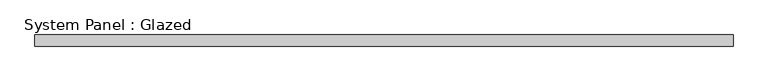
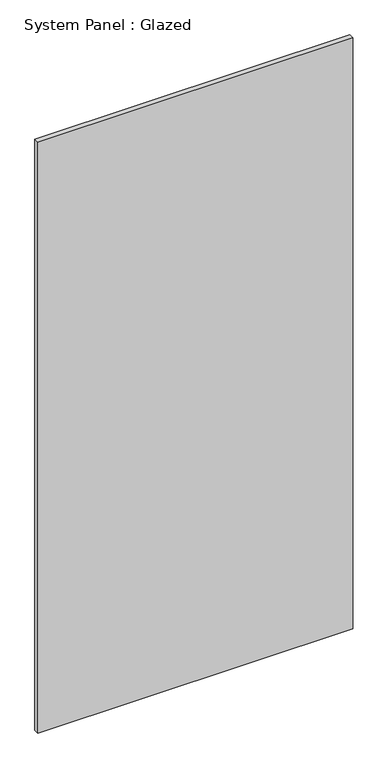
"""IFC4 building model written with IfcOpenShell, lengths in millimetres: plate geometry, System Panel : Glazed."""

from ifc_helpers import new_model, si_unit, origin, origin_with_axes, place, context, project, spatial, polyline, outline, extrude, source, transform, mapped, element, save


def system_panel_glazed_de536e8c(model_context):
    return source(origin(), model_context, "Body", "SweptSolid", [
        extrude(outline(polyline([(756.5339363, 24.5), (-756.5339363, 24.5), (-756.5339363, 49.5), (756.5339363, 49.5), (756.5339363, 24.5)])), origin_with_axes(), (0.0, 0.0, 1.0), 3000.0),
    ])


if __name__ == "__main__":
    model = new_model("IFC4")
    model_context = context("Model", 3, world=origin())
    ifc_project = project(units=[si_unit("LENGTHUNIT", "METRE", prefix="MILLI")], contexts=[model_context])
    site = spatial("IfcSite", under=ifc_project)
    building = spatial("IfcBuilding", under=site)
    placement = place(None, origin())
    system_panel_glazed_shape = system_panel_glazed_de536e8c(model_context)
    element("IfcPlate", 1, ObjectType="System Panel : Glazed", at=placement, inside=building, context=model_context, shape_type="MappedRepresentation", body=[
        mapped(system_panel_glazed_shape, transform((0.0, 0.0, 0.0), x_axis=(1.0, 0.0, 0.0), y_axis=(0.0, 1.0, 0.0), z_axis=(0.0, 0.0, 1.0))),
    ])
    save(model, "model.ifc")

# Revit data of these elements
# Type "System Panel : Glazed"
#   Keynote = "H11"
#   Construction Type Id = "GSP4R"
#   Analytic Construction = "1/8 in Pilkington single glazing"
#   Visual Light Transmittance = 0.9
#   Solar Heat Gain Coefficient = 0.86
#   Heat Transfer Coefficient (U) = 6.7069 W/(m²·K)
#   Define Thermal Properties by = 1
# Element 1 (IfcPlate, "System Panel : Glazed")
#   Materials on its faces: "Glass"
# Materials
#   "Glass": class "Glass", colour RGB 0 128 192, transparency 0.9, Description = "Soda Lime Glass", Cost = 0
